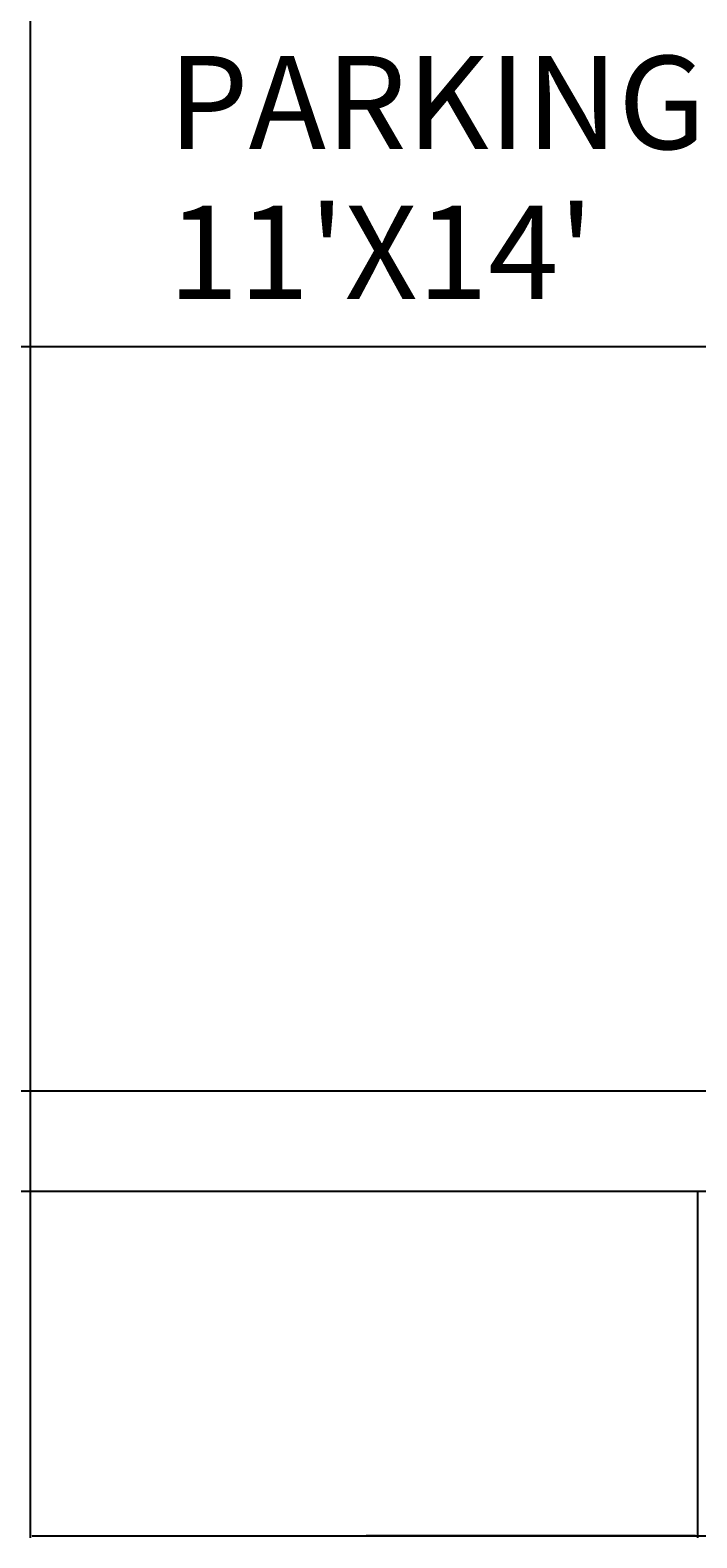
# Model space of a CAD drawing. Units: feet. Extents: x 1654 to 2985, y 1348 to 2230.
# Tile 17 of 53: x 2070 to 2130, y 1534 to 1670. Entities that reach past the tile are written whole.
import ezdxf

# ---------------------------------------------------------------- set-up
doc = ezdxf.new("R2010")
doc.units = ezdxf.units.FT
for name, color, linetype, lineweight in [('A-ANNO-DIMS', 2, 'Continuous', 18), ('A-AREA-IDEN', 7, 'Continuous', 18), ('A-FLOR', 7, 'Continuous', 25)]:
    doc.layers.add(name, color=color, linetype=linetype, lineweight=lineweight)
doc.styles.get("Standard").update_dxf_attribs({"font": 'arial.ttf'})
doc.dimstyles.get("Standard").update_dxf_attribs({"dimtxt": 0.18, "dimasz": 0.18, "dimexe": 0.18, "dimexo": 0.0625, "dimgap": 0.09, "dimtad": 0, "dimtih": 1, "dimtoh": 1, "dimdec": 4, "dimzin": 0, "dimdsep": 46, "dimtxsty": 'Standard', "dimcen": 0.09, "dimadec": 0, "dimazin": 0, "dimtfac": 1, "dimtdec": 4, "dimtofl": 0, "dimtmove": 0, "dimatfit": 3, "dimfxl": 1, "dimtolj": 1, "dimtzin": 0, "dimarcsym": 0})

# ---------------------------------------------------------------- blocks, each defined once
blk = doc.blocks.new('*D80')
at = {"layer": 'A-ANNO-DIMS', "color": 0, "lineweight": -2, "transparency": 16777216}
for p, q in [((2070.09, 2039.19), (2070.09, 1534.07)), ((2202.09, 2039.19), (2202.09, 1534.07)), ((2070.27, 1534.25), (2135.81, 1534.25)), ((2201.91, 1534.25), (2136.37, 1534.25))]:
    blk.add_line(p, q, dxfattribs=at)
at = {"layer": 'A-ANNO-DIMS', "color": 0, "transparency": 16777216}
for points in [[(2070.27, 1534.28), (2070.27, 1534.22), (2070.09, 1534.25)], [(2201.91, 1534.28), (2201.91, 1534.22), (2202.09, 1534.25)]]:
    blk.add_solid(points, dxfattribs=at)
at = {"layer": 'Defpoints', "color": 0, "transparency": 16777216}
for p in [(2070.09, 2039.25), (2202.09, 2039.25), (2202.09, 1534.25)]:
    blk.add_point(p, dxfattribs=at)
at = {"layer": 'A-ANNO-DIMS', "color": 0, "transparency": 16777216, "insert": (2136.09, 1534.25), "char_height": 0.18, "attachment_point": 5}
blk.add_mtext('\\A1;132', dxfattribs=at)
blk = doc.blocks.new('*D90')
at = {"layer": 'A-ANNO-DIMS', "color": 0, "lineweight": -2, "transparency": 16777216}
for p, q in [((1852.15, 1641.19), (2242.27, 1641.19)), ((2242.09, 1641.01), (2242.09, 1607.9)), ((2242.09, 1574.43), (2242.09, 1607.54)), ((1852.15, 1574.25), (2242.27, 1574.25))]:
    blk.add_line(p, q, dxfattribs=at)
at = {"layer": 'A-ANNO-DIMS', "color": 0, "transparency": 16777216}
for points in [[(2242.06, 1641.01), (2242.12, 1641.01), (2242.09, 1641.19)], [(2242.06, 1574.43), (2242.12, 1574.43), (2242.09, 1574.25)]]:
    blk.add_solid(points, dxfattribs=at)
at = {"layer": 'Defpoints', "color": 0, "transparency": 16777216}
for p in [(1852.09, 1641.19), (2242.09, 1641.19), (1852.09, 1574.25)]:
    blk.add_point(p, dxfattribs=at)
at = {"layer": 'A-ANNO-DIMS', "color": 0, "transparency": 16777216, "insert": (2242.09, 1607.72), "char_height": 0.18, "attachment_point": 5}
blk.add_mtext('\\A1;66.93', dxfattribs=at)
blk = doc.blocks.new('*D103')
at = {"layer": 'A-ANNO-DIMS', "color": 0, "lineweight": -2, "transparency": 16777216}
for p, q in [((2070.09, 1661.19), (2070.09, 1534.07)), ((2130.09, 1565.19), (2130.09, 1534.07)), ((2070.27, 1534.25), (2099.87, 1534.25)), ((2129.91, 1534.25), (2100.31, 1534.25))]:
    blk.add_line(p, q, dxfattribs=at)
at = {"layer": 'A-ANNO-DIMS', "color": 0, "transparency": 16777216}
for points in [[(2070.27, 1534.28), (2070.27, 1534.22), (2070.09, 1534.25)], [(2129.91, 1534.28), (2129.91, 1534.22), (2130.09, 1534.25)]]:
    blk.add_solid(points, dxfattribs=at)
at = {"layer": 'Defpoints', "color": 0, "transparency": 16777216}
for p in [(2070.09, 1661.25), (2130.09, 1565.25), (2130.09, 1534.25)]:
    blk.add_point(p, dxfattribs=at)
at = {"layer": 'A-ANNO-DIMS', "color": 0, "transparency": 16777216, "insert": (2100.09, 1534.25), "char_height": 0.18, "attachment_point": 5}
blk.add_mtext('\\A1;60', dxfattribs=at)

msp = doc.modelspace()

# ---------------------------------------------------------------- linework, layer by layer
at = {"layer": 'A-FLOR'}
msp.add_line((2008.0924, 1565.2549), (2211.0924, 1565.2549), dxfattribs=at)

# ---------------------------------------------------------------- texts
at = {"layer": 'A-AREA-IDEN'}
for s, p in [('PARKING', (2082.497, 1658.9308)), ("11'X14'", (2082.497, 1645.4672))]:
    msp.add_text(s, height=8.38114, dxfattribs=at).set_placement(p)

# ---------------------------------------------------------------- dimensions: what is measured, and where the dimension line sits
at = {"layer": 'A-ANNO-DIMS'}
for base, p1, p2, picture, middle in [((2202.0924, 1534.2549), (2070.0924, 2039.2549), (2202.0924, 2039.2549), '*D80', (2136.0924, 1534.2549)), ((2130.0924, 1534.2549), (2070.0924, 1661.2549), (2130.0924, 1565.2549), '*D103', (2100.0924, 1534.2549))]:
    dim = msp.add_linear_dim(base=base, p1=p1, p2=p2, dimstyle='Standard', override={"dimdec": 0, "dimlfac": 1, "dimrnd": 0, "dimzin": 0, "dimdsep": 46, "dimlunit": 2}, dxfattribs=at)
    dim.commit()
    dim.dimension.update_dxf_attribs({"geometry": picture, "text_midpoint": middle})
dim = msp.add_linear_dim(base=(2242.0924, 1641.187), p1=(1852.0924, 1574.2549), p2=(1852.0924, 1641.187), angle=90, dimstyle='Standard', override={"dimdec": 2, "dimlfac": 1, "dimrnd": 0, "dimzin": 0, "dimdsep": 46, "dimlunit": 2}, dxfattribs=at)
dim.commit()
dim.dimension.update_dxf_attribs({"geometry": '*D90', "text_midpoint": (2242.0924, 1607.721)})

doc.saveas('drawing.dxf')
